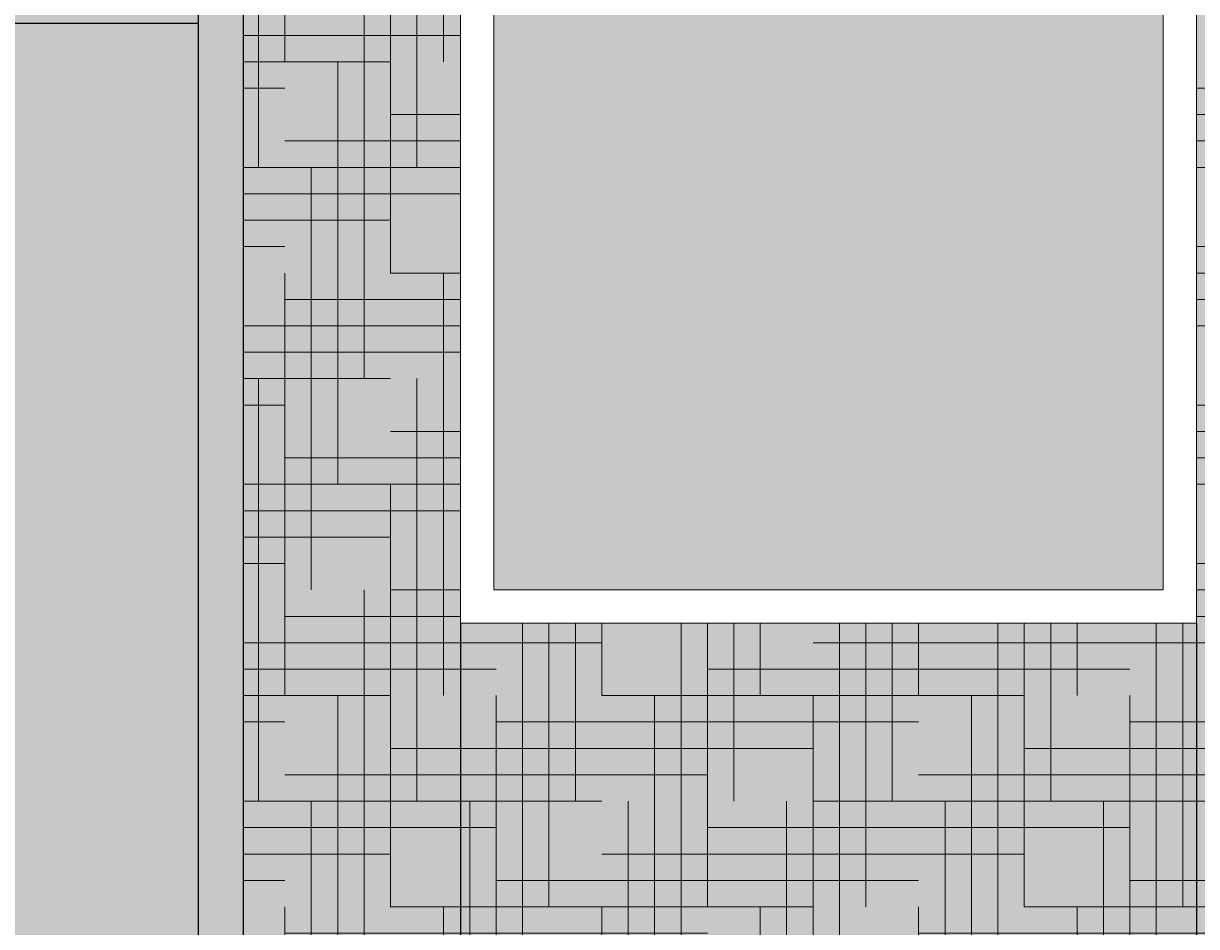
# Model space of a CAD drawing. Units: inches. Extents: x 3024 to 4744, y 1110 to 2100.
# Tile 10 of 29: x 3309 to 3450, y 1293 to 1402. Entities that reach past the tile are written whole.
import ezdxf

# ---------------------------------------------------------------- set-up
doc = ezdxf.new("R2010")
doc.units = ezdxf.units.IN
for name, color, linetype, lineweight in [('A-ANNO-DIMS', 2, 'Continuous', 18), ('A-ELEV', 7, 'Continuous', 25), ('A-ELEV-PATT', 252, 'Continuous', 13), ('A-GLAZ', 4, 'Continuous', 18)]:
    doc.layers.add(name, color=color, linetype=linetype, lineweight=lineweight)
doc.styles.get("Standard").update_dxf_attribs({"font": 'arial.ttf'})
doc.dimstyles.get("Standard").update_dxf_attribs({"dimtxt": 0.18, "dimasz": 0.18, "dimexe": 0.18, "dimexo": 0.0625, "dimgap": 0.09, "dimtad": 0, "dimtih": 1, "dimtoh": 1, "dimdec": 1, "dimzin": 0, "dimdsep": 46, "dimlunit": 3, "dimtxsty": 'Standard', "dimcen": 0.09, "dimadec": 0, "dimazin": 0, "dimtfac": 1, "dimtdec": 1, "dimtofl": 0, "dimtmove": 0, "dimatfit": 3, "dimfxl": 1, "dimtolj": 1, "dimtzin": 0, "dimarcsym": 0})

# ---------------------------------------------------------------- blocks, each defined once
blk = doc.blocks.new('WIN-STONE-CENTRE')
for points in [[(3361.22, 1940.61), (3449.72, 1940.61), (3449.72, 1833.52), (3361.22, 1833.52)], [(3361.22, 1940.61), (3449.72, 1940.61), (3449.72, 1833.52), (3361.22, 1833.52)], [(3365.22, 1936.61), (3445.72, 1936.61), (3445.72, 1837.52), (3365.22, 1837.52)], [(3365.22, 1936.61), (3445.72, 1936.61), (3445.72, 1837.52), (3365.22, 1837.52)]]:
    blk.add_lwpolyline(points, close=True)
blk = doc.blocks.new('*D56')
at = {"layer": 'A-ANNO-DIMS', "color": 0, "lineweight": -2, "transparency": 16777216}
for p, q in [((3361.22, 1329.46), (3361.22, 1109.93)), ((3329.7, 1155.55), (3329.7, 1109.93)), ((3329.88, 1110.11), (3345.07, 1110.11)), ((3361.04, 1110.11), (3345.86, 1110.11))]:
    blk.add_line(p, q, dxfattribs=at)
at = {"layer": 'A-ANNO-DIMS', "color": 0, "transparency": 16777216}
for points in [[(3329.88, 1110.14), (3329.88, 1110.08), (3329.7, 1110.11)], [(3361.04, 1110.14), (3361.04, 1110.08), (3361.22, 1110.11)]]:
    blk.add_solid(points, dxfattribs=at)
at = {"layer": 'Defpoints', "color": 0, "transparency": 16777216}
for p in [(3361.22, 1329.52), (3329.7, 1155.61), (3361.22, 1110.11)]:
    blk.add_point(p, dxfattribs=at)
at = {"layer": 'A-ANNO-DIMS', "color": 0, "transparency": 16777216, "insert": (3345.46, 1110.11), "char_height": 0.18, "attachment_point": 5}
blk.add_mtext('\\A1;31.52', dxfattribs=at)
blk = doc.blocks.new('*D57')
at = {"layer": 'A-ANNO-DIMS', "color": 0, "lineweight": -2, "transparency": 16777216}
for p, q in [((3361.22, 1329.46), (3361.22, 1109.93)), ((3449.72, 1329.46), (3449.72, 1109.93)), ((3361.4, 1110.11), (3405.15, 1110.11)), ((3449.54, 1110.11), (3405.8, 1110.11))]:
    blk.add_line(p, q, dxfattribs=at)
at = {"layer": 'A-ANNO-DIMS', "color": 0, "transparency": 16777216}
for points in [[(3361.4, 1110.14), (3361.4, 1110.08), (3361.22, 1110.11)], [(3449.54, 1110.14), (3449.54, 1110.08), (3449.72, 1110.11)]]:
    blk.add_solid(points, dxfattribs=at)
at = {"layer": 'Defpoints', "color": 0, "transparency": 16777216}
for p in [(3361.22, 1329.52), (3449.72, 1329.52), (3449.72, 1110.11)]:
    blk.add_point(p, dxfattribs=at)
at = {"layer": 'A-ANNO-DIMS', "color": 0, "transparency": 16777216, "insert": (3405.47, 1110.11), "char_height": 0.18, "attachment_point": 5}
blk.add_mtext('\\A1;88.5', dxfattribs=at)
blk = doc.blocks.new('*D64')
at = {"layer": 'A-ANNO-DIMS', "color": 0, "lineweight": -2, "transparency": 16777216}
for p, q in [((3069.79, 1241.5), (3069.79, 2100.44)), ((3069.97, 2100.26), (3405.08, 2100.26)), ((3740.97, 2100.26), (3405.87, 2100.26)), ((3741.15, 1241.5), (3741.15, 2100.44))]:
    blk.add_line(p, q, dxfattribs=at)
at = {"layer": 'A-ANNO-DIMS', "color": 0, "transparency": 16777216}
for points in [[(3069.97, 2100.29), (3069.97, 2100.23), (3069.79, 2100.26)], [(3740.97, 2100.29), (3740.97, 2100.23), (3741.15, 2100.26)]]:
    blk.add_solid(points, dxfattribs=at)
at = {"layer": 'Defpoints', "color": 0, "transparency": 16777216}
for p in [(3741.15, 2100.26), (3069.79, 1241.43), (3741.15, 1241.43)]:
    blk.add_point(p, dxfattribs=at)
at = {"layer": 'A-ANNO-DIMS', "color": 0, "transparency": 16777216, "insert": (3405.47, 2100.26), "char_height": 0.18, "attachment_point": 5}
blk.add_mtext('\\A1;671.4', dxfattribs=at)

msp = doc.modelspace()

# ---------------------------------------------------------------- hatches: boundary and pattern name
at = {"layer": 'A-ELEV-PATT'}
h = msp.add_hatch(color=256, dxfattribs=at)
h.dxf.hatch_style = 1
h.paths.add_polyline_path([(3335.1044, 2043.5286), (3329.7033, 2043.5286), (3329.7033, 1155.6112), (3335.1044, 1155.6112)])
h.paths.add_polyline_path([(3481.2411, 2043.5286), (3335.1044, 2043.5286), (3335.1044, 1155.6112), (3481.2411, 1155.6112)])
h.paths.add_polyline_path([(3449.7202, 1329.5246), (3361.2242, 1329.5246), (3361.2242, 1436.6064), (3449.7202, 1436.6064)], flags=16)
h.paths.add_polyline_path([(3445.7202, 1333.5246), (3365.2242, 1333.5246), (3365.2242, 1432.6064), (3445.7202, 1432.6064)], flags=0)
h.paths.add_polyline_path([(3449.7202, 1455.5246), (3361.2242, 1455.5246), (3361.2242, 1562.6064), (3449.7202, 1562.6064)], flags=16)
h.paths.add_polyline_path([(3445.7202, 1459.5246), (3365.2242, 1459.5246), (3365.2242, 1558.6064), (3445.7202, 1558.6064)], flags=0)
h.paths.add_polyline_path([(3449.7202, 1581.5246), (3361.2242, 1581.5246), (3361.2242, 1688.6064), (3449.7202, 1688.6064)], flags=16)
h.paths.add_polyline_path([(3445.7202, 1585.5246), (3365.2242, 1585.5246), (3365.2242, 1684.6064), (3445.7202, 1684.6064)], flags=0)
h.paths.add_polyline_path([(3449.7202, 1707.5246), (3361.2242, 1707.5246), (3361.2242, 1814.6064), (3449.7202, 1814.6064)], flags=16)
h.paths.add_polyline_path([(3445.7202, 1711.5246), (3365.2242, 1711.5246), (3365.2242, 1810.6064), (3445.7202, 1810.6064)], flags=0)
h.paths.add_polyline_path([(3449.7202, 1833.5246), (3361.2242, 1833.5246), (3361.2242, 1940.6064), (3449.7202, 1940.6064)], flags=16)
h.paths.add_polyline_path([(3445.7202, 1837.5246), (3365.2242, 1837.5246), (3365.2242, 1936.6064), (3445.7202, 1936.6064)], flags=0)
h = msp.add_hatch(color=256, dxfattribs=at)
h.dxf.hatch_style = 1
h.paths.add_polyline_path([(3475.84, 2043.5286), (3335.1044, 2043.5286), (3335.1044, 1155.6112), (3475.84, 1155.6112)])
h.paths.add_polyline_path([(3449.7202, 1940.6064), (3449.7202, 1833.5246), (3361.2242, 1833.5246), (3361.2242, 1940.6064)], flags=16)
h.paths.add_polyline_path([(3445.7202, 1936.6064), (3445.7202, 1837.5246), (3365.2242, 1837.5246), (3365.2242, 1936.6064)], flags=0)
h.paths.add_polyline_path([(3449.7202, 1814.6064), (3449.7202, 1707.5246), (3361.2242, 1707.5246), (3361.2242, 1814.6064)], flags=16)
h.paths.add_polyline_path([(3445.7202, 1810.6064), (3445.7202, 1711.5246), (3365.2242, 1711.5246), (3365.2242, 1810.6064)], flags=0)
h.paths.add_polyline_path([(3449.7202, 1688.6064), (3449.7202, 1581.5246), (3361.2242, 1581.5246), (3361.2242, 1688.6064)], flags=16)
h.paths.add_polyline_path([(3445.7202, 1684.6064), (3445.7202, 1585.5246), (3365.2242, 1585.5246), (3365.2242, 1684.6064)], flags=0)
h.paths.add_polyline_path([(3449.7202, 1562.6064), (3449.7202, 1455.5246), (3361.2242, 1455.5246), (3361.2242, 1562.6064)], flags=16)
h.paths.add_polyline_path([(3445.7202, 1558.6064), (3445.7202, 1459.5246), (3365.2242, 1459.5246), (3365.2242, 1558.6064)], flags=0)
h.paths.add_polyline_path([(3449.7202, 1436.6064), (3449.7202, 1329.5246), (3361.2242, 1329.5246), (3361.2242, 1436.6064)], flags=16)
h.paths.add_polyline_path([(3445.7202, 1432.6064), (3445.7202, 1333.5246), (3365.2242, 1333.5246), (3365.2242, 1432.6064)], flags=0)
h = msp.add_hatch(dxfattribs=at)
h.set_pattern_fill('HOUND', color=256, scale=2)
h.paths.add_polyline_path([(3475.84, 2043.5286), (3335.1044, 2043.5286), (3335.1044, 1155.6112), (3475.84, 1155.6112)])
h.paths.add_polyline_path([(3449.7202, 1940.6064), (3449.7202, 1833.5246), (3361.2242, 1833.5246), (3361.2242, 1940.6064)], flags=16)
h.paths.add_polyline_path([(3445.7202, 1936.6064), (3445.7202, 1837.5246), (3365.2242, 1837.5246), (3365.2242, 1936.6064)], flags=0)
h.paths.add_polyline_path([(3449.7202, 1814.6064), (3449.7202, 1707.5246), (3361.2242, 1707.5246), (3361.2242, 1814.6064)], flags=16)
h.paths.add_polyline_path([(3445.7202, 1810.6064), (3445.7202, 1711.5246), (3365.2242, 1711.5246), (3365.2242, 1810.6064)], flags=0)
h.paths.add_polyline_path([(3449.7202, 1688.6064), (3449.7202, 1581.5246), (3361.2242, 1581.5246), (3361.2242, 1688.6064)], flags=16)
h.paths.add_polyline_path([(3445.7202, 1684.6064), (3445.7202, 1585.5246), (3365.2242, 1585.5246), (3365.2242, 1684.6064)], flags=0)
h.paths.add_polyline_path([(3449.7202, 1562.6064), (3449.7202, 1455.5246), (3361.2242, 1455.5246), (3361.2242, 1562.6064)], flags=16)
h.paths.add_polyline_path([(3445.7202, 1558.6064), (3445.7202, 1459.5246), (3365.2242, 1459.5246), (3365.2242, 1558.6064)], flags=0)
h.paths.add_polyline_path([(3449.7202, 1436.6064), (3449.7202, 1329.5246), (3361.2242, 1329.5246), (3361.2242, 1436.6064)], flags=16)
h.paths.add_polyline_path([(3445.7202, 1432.6064), (3445.7202, 1333.5246), (3365.2242, 1333.5246), (3365.2242, 1432.6064)], flags=0)
h = msp.add_hatch(color=256, dxfattribs=at)
h.dxf.hatch_style = 1
h.paths.add_polyline_path([(3445.7202, 1936.6064), (3365.2242, 1936.6064), (3365.2242, 1837.5246), (3445.7202, 1837.5246)])
h.paths.add_polyline_path([(3445.7202, 1810.6064), (3365.2242, 1810.6064), (3365.2242, 1711.5246), (3445.7202, 1711.5246)])
h.paths.add_polyline_path([(3445.7202, 1684.6064), (3365.2242, 1684.6064), (3365.2242, 1585.5246), (3445.7202, 1585.5246)])
h.paths.add_polyline_path([(3445.7202, 1558.6064), (3365.2242, 1558.6064), (3365.2242, 1459.5246), (3445.7202, 1459.5246)])
h.paths.add_polyline_path([(3445.7202, 1432.6064), (3365.2242, 1432.6064), (3365.2242, 1333.5246), (3445.7202, 1333.5246)])
h = msp.add_hatch(color=256, dxfattribs=at)
h.dxf.hatch_style = 1
h.paths.add_polyline_path([(3329.7033, 1407.6112), (3105.4722, 1407.6112), (3105.4722, 1401.6112), (3329.7033, 1401.6112)])
h.paths.add_polyline_path([(3329.7033, 1281.6112), (3105.4722, 1281.6112), (3105.4722, 1275.6112), (3112.3838, 1275.6112), (3329.7033, 1275.6112)])
h.paths.add_polyline_path([(3329.7033, 1533.6112), (3105.4722, 1533.6112), (3105.4722, 1527.6112), (3329.7033, 1527.6112)])
h.paths.add_polyline_path([(3329.7033, 1659.6112), (3105.4722, 1659.6112), (3105.4722, 1653.6112), (3329.7033, 1653.6112)])
h.paths.add_polyline_path([(3329.7033, 1785.6112), (3105.4722, 1785.6112), (3105.4722, 1779.6112), (3329.7033, 1779.6112)])
h.paths.add_polyline_path([(3329.7033, 1911.6112), (3105.4722, 1911.6112), (3095.7158, 1911.6112), (3095.7158, 1905.6112), (3329.7033, 1905.6112)])
h.paths.add_polyline_path([(3715.2286, 1911.6112), (3705.4722, 1911.6112), (3705.4722, 1905.6112), (3715.2286, 1905.6112)])
h.paths.add_polyline_path([(3688.5588, 1911.6112), (3481.2411, 1911.6112), (3481.2411, 1905.6112), (3688.5588, 1905.6112)])
h = msp.add_hatch(color=256, dxfattribs=at)
h.dxf.hatch_style = 1
h.paths.add_polyline_path([(3154.3287, 1897.4879), (3148.9694, 1897.4879), (3148.9694, 1905.6112), (3105.4722, 1905.6112), (3105.4722, 1785.6112), (3148.9694, 1785.6112), (3148.9694, 1795.0431), (3151.6604, 1795.0431), (3151.6604, 1806.8674), (3154.3287, 1806.8674)])
h.paths.add_polyline_path([(3329.7033, 1905.6112), (3292.6051, 1905.6112), (3292.6051, 1897.4879), (3287.2458, 1897.4879), (3287.2458, 1806.8674), (3288.3759, 1806.8674), (3288.3759, 1795.0431), (3292.6051, 1795.0431), (3292.6051, 1785.6112), (3329.7033, 1785.6112)])
h.paths.add_polyline_path([(3154.3287, 1771.4879), (3148.9694, 1771.4879), (3148.9694, 1779.6112), (3105.4722, 1779.6112), (3105.4722, 1659.6112), (3148.9694, 1659.6112), (3148.9694, 1669.0431), (3151.6604, 1669.0431), (3151.6604, 1680.8674), (3154.3287, 1680.8674)])
h.paths.add_polyline_path([(3329.7033, 1779.6112), (3292.6051, 1779.6112), (3292.6051, 1771.4879), (3287.2458, 1771.4879), (3287.2458, 1680.8674), (3288.3759, 1680.8674), (3288.3759, 1669.0431), (3292.6051, 1669.0431), (3292.6051, 1659.6112), (3329.7033, 1659.6112)])
h.paths.add_polyline_path([(3154.3287, 1645.4879), (3148.9694, 1645.4879), (3148.9694, 1653.6112), (3105.4722, 1653.6112), (3105.4722, 1533.6112), (3148.9694, 1533.6112), (3148.9694, 1543.0431), (3151.6604, 1543.0431), (3151.6604, 1554.8674), (3154.3287, 1554.8674)])
h.paths.add_polyline_path([(3329.7033, 1653.6112), (3292.6051, 1653.6112), (3292.6051, 1645.4879), (3287.2458, 1645.4879), (3287.2458, 1554.8674), (3288.3759, 1554.8674), (3288.3759, 1543.0431), (3292.6051, 1543.0431), (3292.6051, 1533.6112), (3329.7033, 1533.6112)])
h.paths.add_polyline_path([(3329.7033, 1527.6112), (3292.6051, 1527.6112), (3292.6051, 1519.4879), (3287.2458, 1519.4879), (3287.2458, 1428.8674), (3288.3759, 1428.8674), (3288.3759, 1417.0431), (3292.6051, 1417.0431), (3292.6051, 1407.6112), (3329.7033, 1407.6112)])
h.paths.add_polyline_path([(3329.7033, 1401.6112), (3292.6051, 1401.6112), (3292.6051, 1393.4879), (3287.2458, 1393.4879), (3287.2458, 1302.8674), (3288.3759, 1302.8674), (3288.3759, 1291.0431), (3292.6051, 1291.0431), (3292.6051, 1281.6112), (3329.7033, 1281.6112)])
h.paths.add_polyline_path([(3154.3287, 1393.4879), (3148.9694, 1393.4879), (3148.9694, 1401.6112), (3105.4722, 1401.6112), (3105.4722, 1281.6112), (3148.9694, 1281.6112), (3148.9694, 1291.0431), (3151.6604, 1291.0431), (3151.6604, 1302.8674), (3154.3287, 1302.8674)])
h.paths.add_polyline_path([(3154.3287, 1519.4879), (3148.9694, 1519.4879), (3148.9694, 1527.6112), (3105.4722, 1527.6112), (3105.4722, 1407.6112), (3148.9694, 1407.6112), (3148.9694, 1417.0431), (3151.6604, 1417.0431), (3151.6604, 1428.8674), (3154.3287, 1428.8674)])
h.paths.add_polyline_path([(3515.7606, 1897.4879), (3510.4013, 1897.4879), (3510.4013, 1905.6112), (3481.2411, 1905.6112), (3481.2411, 1785.6112), (3510.4013, 1785.6112), (3510.4013, 1795.0431), (3513.0923, 1795.0431), (3513.0923, 1806.8674), (3515.7606, 1806.8674)])
h.paths.add_polyline_path([(3688.5588, 1905.6112), (3654.037, 1905.6112), (3654.037, 1897.4879), (3648.6777, 1897.4879), (3648.6777, 1806.8674), (3649.8078, 1806.8674), (3649.8078, 1795.0431), (3654.037, 1795.0431), (3654.037, 1785.6112), (3688.5588, 1785.6112)])
h.paths.add_polyline_path([(3515.7606, 1771.4879), (3510.4013, 1771.4879), (3510.4013, 1779.6112), (3481.2411, 1779.6112), (3481.2411, 1659.6112), (3510.4013, 1659.6112), (3510.4013, 1669.0431), (3513.0923, 1669.0431), (3513.0923, 1680.8674), (3515.7606, 1680.8674)])
h.paths.add_polyline_path([(3688.5588, 1779.6112), (3654.037, 1779.6112), (3654.037, 1771.4879), (3648.6777, 1771.4879), (3648.6777, 1680.8674), (3649.8078, 1680.8674), (3649.8078, 1669.0431), (3654.037, 1669.0431), (3654.037, 1659.6112), (3688.5588, 1659.6112)])
h.paths.add_polyline_path([(3515.7606, 1645.4879), (3510.4013, 1645.4879), (3510.4013, 1653.6112), (3481.2411, 1653.6112), (3481.2411, 1533.6112), (3510.4013, 1533.6112), (3510.4013, 1543.0431), (3513.0923, 1543.0431), (3513.0923, 1554.8674), (3515.7606, 1554.8674)])
h.paths.add_polyline_path([(3688.5588, 1653.6112), (3654.037, 1653.6112), (3654.037, 1645.4879), (3648.6777, 1645.4879), (3648.6777, 1554.8674), (3649.8078, 1554.8674), (3649.8078, 1543.0431), (3654.037, 1543.0431), (3654.037, 1533.6112), (3688.5588, 1533.6112)])
h.paths.add_polyline_path([(3515.7606, 1519.4879), (3510.4013, 1519.4879), (3510.4013, 1527.6112), (3481.2411, 1527.6112), (3481.2411, 1407.6112), (3510.4013, 1407.6112), (3510.4013, 1417.0431), (3513.0923, 1417.0431), (3513.0923, 1428.8674), (3515.7606, 1428.8674)])
h.paths.add_polyline_path([(3688.5588, 1527.6112), (3654.037, 1527.6112), (3654.037, 1519.4879), (3648.6777, 1519.4879), (3648.6777, 1428.8674), (3649.8078, 1428.8674), (3649.8078, 1417.0431), (3654.037, 1417.0431), (3654.037, 1407.6112), (3688.5588, 1407.6112)])
h.paths.add_polyline_path([(3515.7606, 1393.4879), (3510.4013, 1393.4879), (3510.4013, 1401.6112), (3481.2411, 1401.6112), (3481.2411, 1281.6112), (3510.4013, 1281.6112), (3510.4013, 1291.0431), (3513.0923, 1291.0431), (3513.0923, 1302.8674), (3515.7606, 1302.8674)])
h.paths.add_polyline_path([(3688.5588, 1401.6112), (3654.037, 1401.6112), (3654.037, 1393.4879), (3648.6777, 1393.4879), (3648.6777, 1302.8674), (3649.8078, 1302.8674), (3649.8078, 1291.0431), (3654.037, 1291.0431), (3654.037, 1281.6112), (3688.5588, 1281.6112)])
h.paths.add_polyline_path([(3515.7606, 1267.4879), (3510.4013, 1267.4879), (3510.4013, 1275.6112), (3481.2411, 1275.6112), (3481.2411, 1155.6112), (3510.4013, 1155.6112), (3510.4013, 1165.0431), (3513.0923, 1165.0431), (3513.0923, 1176.8674), (3515.7606, 1176.8674)])
h.paths.add_polyline_path([(3688.5588, 1275.6112), (3654.037, 1275.6112), (3654.037, 1267.4879), (3648.6777, 1267.4879), (3648.6777, 1176.8674), (3649.8078, 1176.8674), (3649.8078, 1165.0431), (3654.037, 1165.0431), (3654.037, 1155.6112), (3688.5588, 1155.6112)])
h.paths.add_polyline_path([(3112.3838, 1275.6112), (3105.4722, 1275.6112), (3105.4722, 1171.0239), (3112.3838, 1171.0239)])

# ---------------------------------------------------------------- linework, layer by layer
at = {"layer": 'A-ELEV'}
msp.add_line((3329.7033, 1401.6112), (3105.4722, 1401.6112), dxfattribs=at)
msp.add_line((3329.7033, 1401.6112), (3105.4722, 1401.6112), dxfattribs=at)
for points in [[(3481.2411, 1155.6112), (3329.7033, 1155.6112), (3329.7033, 2043.5286), (3481.2411, 2043.5286)], [(3329.7033, 2043.5286), (3335.1044, 2043.5286), (3335.1044, 1155.6112), (3329.7033, 1155.6112)], [(3481.2411, 1155.6112), (3329.7033, 1155.6112), (3329.7033, 2043.5286), (3481.2411, 2043.5286)], [(3329.7033, 2043.5286), (3335.1044, 2043.5286), (3335.1044, 1155.6112), (3329.7033, 1155.6112)]]:
    msp.add_lwpolyline(points, close=True, dxfattribs=at)

# ---------------------------------------------------------------- block references
at = {"layer": 'A-GLAZ'}
msp.add_blockref('WIN-STONE-CENTRE', (0, -504), dxfattribs=at)

# ---------------------------------------------------------------- dimensions: what is measured, and where the dimension line sits
at = {"layer": 'A-ANNO-DIMS'}
for base, p1, p2, override, picture, middle in [((3741.1507, 2100.2584), (3069.7937, 1241.4341), (3741.1507, 1241.4341), {"dimdec": 1, "dimlfac": 1, "dimrnd": 0, "dimzin": 0, "dimdsep": 46, "dimlunit": 2}, '*D64', (3405.4722, 2100.2584)), ((3361.2242, 1110.1112), (3329.7033, 1155.6112), (3361.2242, 1329.5246), {"dimdec": 2, "dimlfac": 1, "dimrnd": 0, "dimzin": 0, "dimdsep": 46, "dimlunit": 2}, '*D56', (3345.4638, 1110.1112)), ((3449.7202, 1110.1112), (3361.2242, 1329.5246), (3449.7202, 1329.5246), {"dimdec": 1, "dimlfac": 1, "dimrnd": 0, "dimzin": 0, "dimdsep": 46, "dimlunit": 2}, '*D57', (3405.4722, 1110.1112))]:
    dim = msp.add_linear_dim(base=base, p1=p1, p2=p2, dimstyle='Standard', override=override, dxfattribs=at)
    dim.commit()
    dim.dimension.update_dxf_attribs({"geometry": picture, "text_midpoint": middle})

doc.saveas('drawing.dxf')
